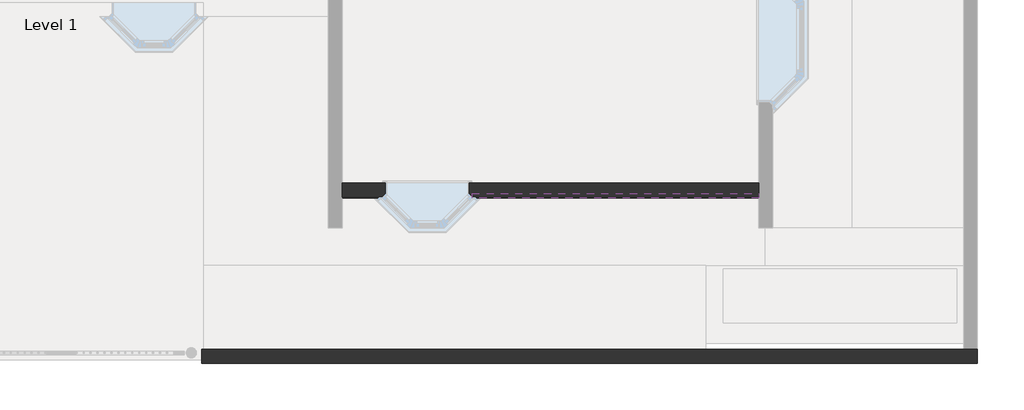
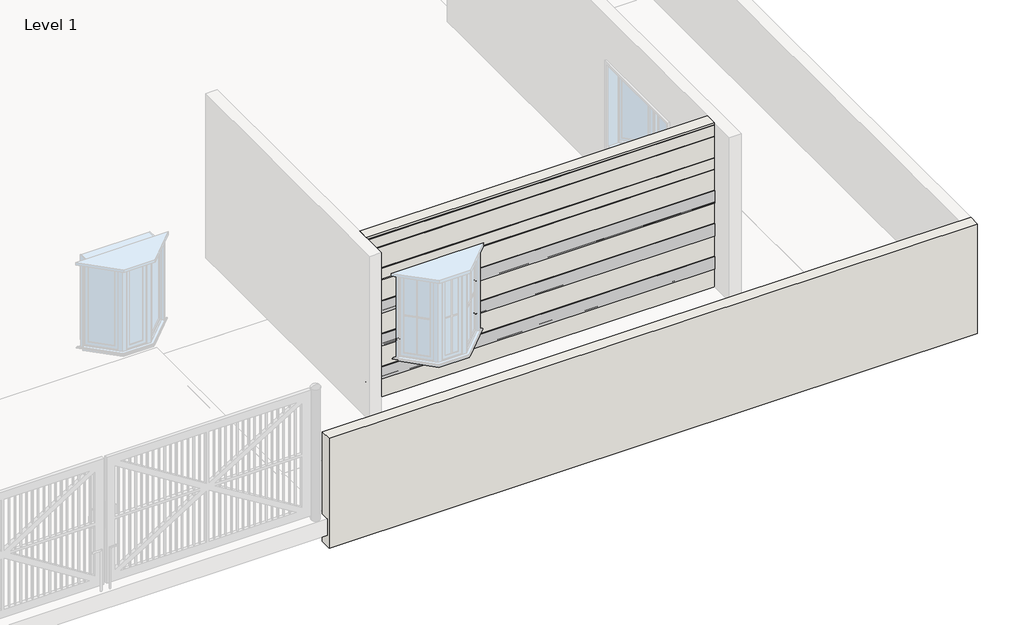
# One storey, part 2 of 5: 3 proxies, 2 walls.
"""IFC4 building model written with IfcOpenShell, lengths in millimetres."""

from ifc_helpers import new_model, si_unit, point, frame, frame_2d, origin, place, context, project, spatial, polyline, circle_curve, ellipse_curve, trimmed, segment, composite_curve, outline, extrude, faceted_brep, element, save
from ifc_brep_helpers import plane_surface, cylinder_surface, revolved_surface, advanced_brep

model = new_model("IFC4")

# Units and contexts
model_context = context("Model", 3, world=origin())
ifc_project = project(units=[si_unit("LENGTHUNIT", "METRE", prefix="MILLI")], contexts=[model_context])

# Site, building, storey
site = spatial("IfcSite", under=ifc_project)
building = spatial("IfcBuilding", under=site)
storey = spatial("IfcBuildingStorey", under=building, Name="Level 1", Elevation=0.0)

# Proxies
placement = place(None, origin())
element("IfcBuildingElementProxy", 1, Name="Reveal", ObjectType="Reveal", at=placement, inside=storey, context=model_context, shape_type="SweptSolid", body=[
    extrude(outline(composite_curve([segment(polyline([(-10015.9757973, 571.5), (-9952.7297973, 571.5), (-9952.7297973, 570.1203242)]), True, "CONTINUOUS"), segment(trimmed(circle_curve(frame_2d((-9957.9748973, 570.1203242)), 5.2451), [point((-9952.7297973, 570.1203242))], [point((-9957.1126065, 564.9465897))], False, "CARTESIAN"), True, "CONTINUOUS"), segment(polyline([(-9957.1126065, 564.9465897), (-9980.7332973, 561.0098), (-9999.9711789, 557.80348)]), True, "CONTINUOUS"), segment(trimmed(circle_curve(frame_2d((-9998.2465973, 547.456011)), 10.4902), [point((-9999.9711789, 557.80348))], [point((-10008.7367973, 547.456011))], True, "CARTESIAN"), True, "CONTINUOUS"), segment(polyline([(-10008.7367973, 547.456011), (-10008.7367973, 366.943989)]), True, "CONTINUOUS"), segment(trimmed(circle_curve(frame_2d((-9998.2465973, 366.943989)), 10.4902), [point((-10008.7367973, 366.943989))], [point((-9999.9711789, 356.59652))], True, "CARTESIAN"), True, "CONTINUOUS"), segment(polyline([(-9999.9711789, 356.59652), (-9980.7332973, 353.3902), (-9957.1126065, 349.4534103)]), True, "CONTINUOUS"), segment(trimmed(circle_curve(frame_2d((-9957.9748973, 344.2796758)), 5.2451), [point((-9957.1126065, 349.4534103))], [point((-9952.7297973, 344.2796758))], False, "CARTESIAN"), True, "CONTINUOUS"), segment(polyline([(-9952.7297973, 344.2796758), (-9952.7297973, 342.9), (-10015.9757973, 342.9), (-10015.9757973, 571.5)]), True, "CONTINUOUS")], self_intersect=False)), frame((-43545.7380314, 0.0, 0.0), z_axis=(1.0, 0.0, 0.0), x_axis=(0.0, 1.0, 0.0)), (0.0, 0.0, 1.0), 6096.0),
])
element("IfcBuildingElementProxy", 2, Name="Reveal", ObjectType="Reveal", at=placement, inside=storey, context=model_context, shape_type="SweptSolid", body=[
    extrude(outline(composite_curve([segment(polyline([(-10015.9757973, 1181.1), (-9952.7297973, 1181.1), (-9952.7297973, 1179.7203242)]), True, "CONTINUOUS"), segment(trimmed(circle_curve(frame_2d((-9957.9748973, 1179.7203242)), 5.2451), [point((-9952.7297973, 1179.7203242))], [point((-9957.1126065, 1174.5465897))], False, "CARTESIAN"), True, "CONTINUOUS"), segment(polyline([(-9957.1126065, 1174.5465897), (-9980.7332973, 1170.6098), (-9999.9711789, 1167.40348)]), True, "CONTINUOUS"), segment(trimmed(circle_curve(frame_2d((-9998.2465973, 1157.056011)), 10.4902), [point((-9999.9711789, 1167.40348))], [point((-10008.7367973, 1157.056011))], True, "CARTESIAN"), True, "CONTINUOUS"), segment(polyline([(-10008.7367973, 1157.056011), (-10008.7367973, 976.543989)]), True, "CONTINUOUS"), segment(trimmed(circle_curve(frame_2d((-9998.2465973, 976.543989)), 10.4902), [point((-10008.7367973, 976.543989))], [point((-9999.9711789, 966.19652))], True, "CARTESIAN"), True, "CONTINUOUS"), segment(polyline([(-9999.9711789, 966.19652), (-9980.7332973, 962.9902), (-9957.1126065, 959.0534103)]), True, "CONTINUOUS"), segment(trimmed(circle_curve(frame_2d((-9957.9748973, 953.8796758)), 5.2451), [point((-9957.1126065, 959.0534103))], [point((-9952.7297973, 953.8796758))], False, "CARTESIAN"), True, "CONTINUOUS"), segment(polyline([(-9952.7297973, 953.8796758), (-9952.7297973, 952.5), (-10015.9757973, 952.5), (-10015.9757973, 1181.1)]), True, "CONTINUOUS")], self_intersect=False)), frame((-41642.1466227, 0.0, 0.0), z_axis=(1.0, 0.0, 0.0), x_axis=(0.0, 1.0, 0.0)), (0.0, 0.0, 1.0), 4192.4085913),
    extrude(outline(composite_curve([segment(polyline([(-10015.9757973, 1181.1), (-9952.7297973, 1181.1), (-9952.7297973, 1179.7203242)]), True, "CONTINUOUS"), segment(trimmed(circle_curve(frame_2d((-9957.9748973, 1179.7203242)), 5.2451), [point((-9952.7297973, 1179.7203242))], [point((-9957.1126065, 1174.5465897))], False, "CARTESIAN"), True, "CONTINUOUS"), segment(polyline([(-9957.1126065, 1174.5465897), (-9980.7332973, 1170.6098), (-9999.9711789, 1167.40348)]), True, "CONTINUOUS"), segment(trimmed(circle_curve(frame_2d((-9998.2465973, 1157.056011)), 10.4902), [point((-9999.9711789, 1167.40348))], [point((-10008.7367973, 1157.056011))], True, "CARTESIAN"), True, "CONTINUOUS"), segment(polyline([(-10008.7367973, 1157.056011), (-10008.7367973, 976.543989)]), True, "CONTINUOUS"), segment(trimmed(circle_curve(frame_2d((-9998.2465973, 976.543989)), 10.4902), [point((-10008.7367973, 976.543989))], [point((-9999.9711789, 966.19652))], True, "CARTESIAN"), True, "CONTINUOUS"), segment(polyline([(-9999.9711789, 966.19652), (-9980.7332973, 962.9902), (-9957.1126065, 959.0534103)]), True, "CONTINUOUS"), segment(trimmed(circle_curve(frame_2d((-9957.9748973, 953.8796758)), 5.2451), [point((-9957.1126065, 959.0534103))], [point((-9952.7297973, 953.8796758))], False, "CARTESIAN"), True, "CONTINUOUS"), segment(polyline([(-9952.7297973, 953.8796758), (-9952.7297973, 952.5), (-10015.9757973, 952.5), (-10015.9757973, 1181.1)]), True, "CONTINUOUS")], self_intersect=False)), frame((-43545.7380314, 0.0, 0.0), z_axis=(1.0, 0.0, 0.0), x_axis=(0.0, 1.0, 0.0)), (0.0, 0.0, 1.0), 585.6085913),
])
element("IfcBuildingElementProxy", 3, Name="Reveal", ObjectType="Reveal", at=placement, inside=storey, context=model_context, shape_type="SweptSolid", body=[
    extrude(outline(composite_curve([segment(polyline([(-10015.9757973, 1790.7), (-9952.7297973, 1790.7), (-9952.7297973, 1789.3203242)]), True, "CONTINUOUS"), segment(trimmed(circle_curve(frame_2d((-9957.9748973, 1789.3203242)), 5.2451), [point((-9952.7297973, 1789.3203242))], [point((-9957.1126065, 1784.1465897))], False, "CARTESIAN"), True, "CONTINUOUS"), segment(polyline([(-9957.1126065, 1784.1465897), (-9980.7332973, 1780.2098), (-9999.9711789, 1777.00348)]), True, "CONTINUOUS"), segment(trimmed(circle_curve(frame_2d((-9998.2465973, 1766.656011)), 10.4902), [point((-9999.9711789, 1777.00348))], [point((-10008.7367973, 1766.656011))], True, "CARTESIAN"), True, "CONTINUOUS"), segment(polyline([(-10008.7367973, 1766.656011), (-10008.7367973, 1586.143989)]), True, "CONTINUOUS"), segment(trimmed(circle_curve(frame_2d((-9998.2465973, 1586.143989)), 10.4902), [point((-10008.7367973, 1586.143989))], [point((-9999.9711789, 1575.79652))], True, "CARTESIAN"), True, "CONTINUOUS"), segment(polyline([(-9999.9711789, 1575.79652), (-9980.7332973, 1572.5902), (-9957.1126065, 1568.6534103)]), True, "CONTINUOUS"), segment(trimmed(circle_curve(frame_2d((-9957.9748973, 1563.4796758)), 5.2451), [point((-9957.1126065, 1568.6534103))], [point((-9952.7297973, 1563.4796758))], False, "CARTESIAN"), True, "CONTINUOUS"), segment(polyline([(-9952.7297973, 1563.4796758), (-9952.7297973, 1562.1), (-10015.9757973, 1562.1), (-10015.9757973, 1790.7)]), True, "CONTINUOUS")], self_intersect=False)), frame((-41642.1466227, 0.0, 0.0), z_axis=(1.0, 0.0, 0.0), x_axis=(0.0, 1.0, 0.0)), (0.0, 0.0, 1.0), 4192.4085913),
    extrude(outline(composite_curve([segment(polyline([(-10015.9757973, 1790.7), (-9952.7297973, 1790.7), (-9952.7297973, 1789.3203242)]), True, "CONTINUOUS"), segment(trimmed(circle_curve(frame_2d((-9957.9748973, 1789.3203242)), 5.2451), [point((-9952.7297973, 1789.3203242))], [point((-9957.1126065, 1784.1465897))], False, "CARTESIAN"), True, "CONTINUOUS"), segment(polyline([(-9957.1126065, 1784.1465897), (-9980.7332973, 1780.2098), (-9999.9711789, 1777.00348)]), True, "CONTINUOUS"), segment(trimmed(circle_curve(frame_2d((-9998.2465973, 1766.656011)), 10.4902), [point((-9999.9711789, 1777.00348))], [point((-10008.7367973, 1766.656011))], True, "CARTESIAN"), True, "CONTINUOUS"), segment(polyline([(-10008.7367973, 1766.656011), (-10008.7367973, 1586.143989)]), True, "CONTINUOUS"), segment(trimmed(circle_curve(frame_2d((-9998.2465973, 1586.143989)), 10.4902), [point((-10008.7367973, 1586.143989))], [point((-9999.9711789, 1575.79652))], True, "CARTESIAN"), True, "CONTINUOUS"), segment(polyline([(-9999.9711789, 1575.79652), (-9980.7332973, 1572.5902), (-9957.1126065, 1568.6534103)]), True, "CONTINUOUS"), segment(trimmed(circle_curve(frame_2d((-9957.9748973, 1563.4796758)), 5.2451), [point((-9957.1126065, 1568.6534103))], [point((-9952.7297973, 1563.4796758))], False, "CARTESIAN"), True, "CONTINUOUS"), segment(polyline([(-9952.7297973, 1563.4796758), (-9952.7297973, 1562.1), (-10015.9757973, 1562.1), (-10015.9757973, 1790.7)]), True, "CONTINUOUS")], self_intersect=False)), frame((-43545.7380314, 0.0, 0.0), z_axis=(1.0, 0.0, 0.0), x_axis=(0.0, 1.0, 0.0)), (0.0, 0.0, 1.0), 585.6085913),
])

# Walls
element("IfcWall", 4, ObjectType="OUTER WALL 8\"", at=placement, inside=storey, context=model_context, shape_type="AdvancedBrep", body=[
    advanced_brep(
    [(-43545.7380314, -10001.0913973, 0.0), (-37449.7380314, -10001.0913973, 0.0), (-37449.7380314, -10001.0913973, 342.9), (-43545.7380314, -10001.0913973, 342.9), (-37449.7380314, -10001.0913973, 3048.0), (-43545.7380314, -10001.0913973, 3048.0), (-43545.7380314, -10001.0913973, 3009.9), (-37449.7380314, -10001.0913973, 3009.9), (-41642.1466227, -10001.0913973, 609.6), (-42960.1294401, -10001.0913973, 609.6), (-42960.1294401, -10001.0913973, 952.5), (-43545.7380314, -10001.0913973, 952.5), (-43545.7380314, -10001.0913973, 571.5), (-37449.7380314, -10001.0913973, 571.5), (-37449.7380314, -10001.0913973, 952.5), (-41642.1466227, -10001.0913973, 952.5), (-37449.7380314, -10001.0913973, 356.84689), (-37449.7380314, -10001.0913973, 557.55311), (-43545.7380314, -10001.0913973, 557.55311), (-43545.7380314, -10001.0913973, 356.84689), (-43545.7380314, -10001.0913973, 1167.15311), (-43545.7380314, -10001.0913973, 966.44689), (-42960.1294401, -10001.0913973, 966.44689), (-42960.1294401, -10001.0913973, 1167.15311), (-37449.7380314, -10001.0913973, 966.44689), (-37449.7380314, -10001.0913973, 1167.15311), (-41642.1466227, -10001.0913973, 1167.15311), (-41642.1466227, -10001.0913973, 966.44689), (-41642.1466227, -10001.0913973, 1181.1), (-37449.7380314, -10001.0913973, 1181.1), (-37449.7380314, -10001.0913973, 1562.1), (-41642.1466227, -10001.0913973, 1562.1), (-43545.7380314, -10001.0913973, 1181.1), (-42960.1294401, -10001.0913973, 1181.1), (-42960.1294401, -10001.0913973, 1562.1), (-43545.7380314, -10001.0913973, 1562.1), (-43545.7380314, -10001.0913973, 1776.75311), (-43545.7380314, -10001.0913973, 1576.04689), (-42960.1294401, -10001.0913973, 1576.04689), (-42960.1294401, -10001.0913973, 1776.75311), (-41642.1466227, -10001.0913973, 1776.75311), (-41642.1466227, -10001.0913973, 1576.04689), (-37449.7380314, -10001.0913973, 1576.04689), (-37449.7380314, -10001.0913973, 1776.75311), (-41642.1466227, -10001.0913973, 1790.7), (-37449.7380314, -10001.0913973, 1790.7), (-37449.7380314, -10001.0913973, 2171.7), (-41642.1466227, -10001.0913973, 2171.7), (-43545.7380314, -10001.0913973, 1790.7), (-42960.1294401, -10001.0913973, 1790.7), (-42960.1294401, -10001.0913973, 2171.7), (-43545.7380314, -10001.0913973, 2171.7), (-43545.7380314, -10001.0913973, 2386.35311), (-43545.7380314, -10001.0913973, 2185.64689), (-37449.7380314, -10001.0913973, 2185.64689), (-37449.7380314, -10001.0913973, 2386.35311), (-43545.7380314, -10001.0913973, 2400.3), (-37449.7380314, -10001.0913973, 2400.3), (-37449.7380314, -10001.0913973, 2781.3), (-43545.7380314, -10001.0913973, 2781.3), (-43545.7380314, -10001.0913973, 2995.95311), (-43545.7380314, -10001.0913973, 2795.24689), (-37449.7380314, -10001.0913973, 2795.24689), (-37449.7380314, -10001.0913973, 2995.95311), (-37449.7380314, -9797.8913973, 0.0), (-43545.7380314, -9797.8913973, 0.0), (-43545.7380314, -9797.8913973, 3048.0), (-37449.7380314, -9797.8913973, 3048.0), (-41691.5380314, -9797.8913973, 2184.4), (-42910.7380314, -9797.8913973, 2184.4), (-42910.7380314, -9797.8913973, 609.6), (-41691.5380314, -9797.8913973, 609.6), (-43545.7380314, -9952.7297973, 342.9), (-43545.7380314, -9952.7297973, 344.2796758), (-43545.7380314, -9957.1126065, 349.4534103), (-43545.7380314, -9999.9711789, 356.59652), (-43545.7380314, -9999.9711789, 557.80348), (-43545.7380314, -9957.1126065, 564.9465897), (-43545.7380314, -9952.7297973, 570.1203242), (-43545.7380314, -9952.7297973, 571.5), (-43545.7380314, -9952.7297973, 952.5), (-43545.7380314, -9952.7297973, 953.8796758), (-43545.7380314, -9957.1126065, 959.0534103), (-43545.7380314, -9999.9711789, 966.19652), (-43545.7380314, -9999.9711789, 1167.40348), (-43545.7380314, -9957.1126065, 1174.5465897), (-43545.7380314, -9952.7297973, 1179.7203242), (-43545.7380314, -9952.7297973, 1181.1), (-43545.7380314, -9952.7297973, 1562.1), (-43545.7380314, -9952.7297973, 1563.4796758), (-43545.7380314, -9957.1126065, 1568.6534103), (-43545.7380314, -9999.9711789, 1575.79652), (-43545.7380314, -9999.9711789, 1777.00348), (-43545.7380314, -9957.1126065, 1784.1465897), (-43545.7380314, -9952.7297973, 1789.3203242), (-43545.7380314, -9952.7297973, 1790.7), (-43545.7380314, -9952.7297973, 2171.7), (-43545.7380314, -9952.7297973, 2173.0796758), (-43545.7380314, -9957.1126065, 2178.2534103), (-43545.7380314, -9999.9711789, 2185.39652), (-43545.7380314, -9999.9711789, 2386.60348), (-43545.7380314, -9957.1126065, 2393.7465897), (-43545.7380314, -9952.7297973, 2398.9203242), (-43545.7380314, -9952.7297973, 2400.3), (-43545.7380314, -9952.7297973, 2781.3), (-43545.7380314, -9952.7297973, 2782.6796758), (-43545.7380314, -9957.1126065, 2787.8534103), (-43545.7380314, -9999.9711789, 2794.99652), (-43545.7380314, -9999.9711789, 2996.20348), (-43545.7380314, -9957.1126065, 3003.3465897), (-43545.7380314, -9952.7297973, 3008.5203242), (-43545.7380314, -9952.7297973, 3009.9), (-37449.7380314, -9952.7297973, 3009.9), (-37449.7380314, -9952.7297973, 3008.5203242), (-37449.7380314, -9957.1126065, 3003.3465897), (-37449.7380314, -9999.9711789, 2996.20348), (-37449.7380314, -9999.9711789, 2794.99652), (-37449.7380314, -9957.1126065, 2787.8534103), (-37449.7380314, -9952.7297973, 2782.6796758), (-37449.7380314, -9952.7297973, 2781.3), (-37449.7380314, -9952.7297973, 2400.3), (-37449.7380314, -9952.7297973, 2398.9203242), (-37449.7380314, -9957.1126065, 2393.7465897), (-37449.7380314, -9999.9711789, 2386.60348), (-37449.7380314, -9999.9711789, 2185.39652), (-37449.7380314, -9957.1126065, 2178.2534103), (-37449.7380314, -9952.7297973, 2173.0796758), (-37449.7380314, -9952.7297973, 2171.7), (-37449.7380314, -9952.7297973, 1790.7), (-37449.7380314, -9952.7297973, 1789.3203242), (-37449.7380314, -9957.1126065, 1784.1465897), (-37449.7380314, -9999.9711789, 1777.00348), (-37449.7380314, -9999.9711789, 1575.79652), (-37449.7380314, -9957.1126065, 1568.6534103), (-37449.7380314, -9952.7297973, 1563.4796758), (-37449.7380314, -9952.7297973, 1562.1), (-37449.7380314, -9952.7297973, 1181.1), (-37449.7380314, -9952.7297973, 1179.7203242), (-37449.7380314, -9957.1126065, 1174.5465897), (-37449.7380314, -9999.9711789, 1167.40348), (-37449.7380314, -9999.9711789, 966.19652), (-37449.7380314, -9957.1126065, 959.0534103), (-37449.7380314, -9952.7297973, 953.8796758), (-37449.7380314, -9952.7297973, 952.5), (-37449.7380314, -9952.7297973, 571.5), (-37449.7380314, -9952.7297973, 570.1203242), (-37449.7380314, -9957.1126065, 564.9465897), (-37449.7380314, -9999.9711789, 557.80348), (-37449.7380314, -9999.9711789, 356.59652), (-37449.7380314, -9957.1126065, 349.4534103), (-37449.7380314, -9952.7297973, 344.2796758), (-37449.7380314, -9952.7297973, 342.9), (-42910.7380314, -9951.6999886, 2184.4), (-41691.5380314, -9951.6999886, 2184.4), (-41649.2459493, -9993.9920708, 2184.4), (-42953.0301136, -9993.9920708, 2184.4), (-41691.5380314, -9951.6999886, 609.6), (-42910.7380314, -9951.6999886, 609.6), (-42916.1506493, -9957.1126065, 2178.2534103), (-42911.7678401, -9952.7297973, 2173.0796758), (-42911.7678401, -9952.7297973, 2171.7), (-41690.5082227, -9952.7297973, 2171.7), (-41690.5082227, -9952.7297973, 2173.0796758), (-41686.1254136, -9957.1126065, 2178.2534103), (-41642.1466227, -9952.7297973, 1179.7203242), (-41642.1466227, -9952.7297973, 1181.1), (-41642.1466227, -9999.9711789, 1167.40348), (-41642.1466227, -9957.1126065, 1174.5465897), (-41642.1466227, -9957.1126065, 959.0534103), (-41642.1466227, -9999.9711789, 966.19652), (-41642.1466227, -9952.7297973, 952.5), (-41642.1466227, -9952.7297973, 953.8796758), (-42960.1294401, -9952.7297973, 953.8796758), (-42960.1294401, -9952.7297973, 952.5), (-42960.1294401, -9999.9711789, 966.19652), (-42960.1294401, -9957.1126065, 959.0534103), (-42960.1294401, -9957.1126065, 1174.5465897), (-42960.1294401, -9999.9711789, 1167.40348), (-42960.1294401, -9952.7297973, 1181.1), (-42960.1294401, -9952.7297973, 1179.7203242), (-41642.1466227, -9952.7297973, 1789.3203242), (-41642.1466227, -9952.7297973, 1790.7), (-41642.1466227, -9999.9711789, 1777.00348), (-41642.1466227, -9957.1126065, 1784.1465897), (-41642.1466227, -9957.1126065, 1568.6534103), (-41642.1466227, -9999.9711789, 1575.79652), (-41642.1466227, -9952.7297973, 1562.1), (-41642.1466227, -9952.7297973, 1563.4796758), (-42960.1294401, -9952.7297973, 1563.4796758), (-42960.1294401, -9952.7297973, 1562.1), (-42960.1294401, -9999.9711789, 1575.79652), (-42960.1294401, -9957.1126065, 1568.6534103), (-42960.1294401, -9957.1126065, 1784.1465897), (-42960.1294401, -9999.9711789, 1777.00348), (-42960.1294401, -9952.7297973, 1790.7), (-42960.1294401, -9952.7297973, 1789.3203242)],
    [
        (0, 1),
        (1, 2),
        (2, 3),
        (3, 0),
        (4, 5),
        (5, 6),
        (6, 7),
        (7, 4),
        (8, 9),
        (9, 10),
        (10, 11),
        (11, 12),
        (12, 13),
        (13, 14),
        (14, 15),
        (15, 8),
        (16, 17),
        (17, 18),
        (18, 19),
        (19, 16),
        (20, 21),
        (21, 22),
        (22, 23),
        (23, 20),
        (24, 25),
        (25, 26),
        (26, 27),
        (27, 24),
        (28, 29),
        (29, 30),
        (30, 31),
        (31, 28),
        (32, 33),
        (33, 34),
        (34, 35),
        (35, 32),
        (36, 37),
        (37, 38),
        (38, 39),
        (39, 36),
        (40, 41),
        (41, 42),
        (42, 43),
        (43, 40),
        (44, 45),
        (45, 46),
        (46, 47),
        (47, 44),
        (48, 49),
        (49, 50),
        (50, 51),
        (51, 48),
        (52, 53),
        (53, 54),
        (54, 55),
        (55, 52),
        (56, 57),
        (57, 58),
        (58, 59),
        (59, 56),
        (60, 61),
        (61, 62),
        (62, 63),
        (63, 60),
        (64, 65),
        (65, 66),
        (66, 67),
        (67, 64),
        (68, 69),
        (69, 70),
        (70, 71),
        (71, 68),
        (0, 65),
        (64, 1),
        (4, 67),
        (66, 5),
        (3, 72),
        (72, 73),
        (73, 74, circle_curve(frame((-43545.7380314, -9957.9748973, 344.2796758), z_axis=(1.0, 0.0, 0.0), x_axis=(0.0, 1.0, 0.0)), 5.2451)),
        (74, 75),
        (75, 19, circle_curve(frame((-43545.7380314, -9998.2465973, 366.943989), z_axis=(-1.0, 0.0, 0.0), x_axis=(0.0, 1.0, 0.0)), 10.4902)),
        (18, 76, circle_curve(frame((-43545.7380314, -9998.2465973, 547.456011), z_axis=(-1.0, 0.0, 0.0), x_axis=(0.0, 1.0, 0.0)), 10.4902)),
        (76, 77),
        (77, 78, circle_curve(frame((-43545.7380314, -9957.9748973, 570.1203242), z_axis=(1.0, 0.0, 0.0), x_axis=(0.0, 1.0, 0.0)), 5.2451)),
        (78, 79),
        (79, 12),
        (11, 80),
        (80, 81),
        (81, 82, circle_curve(frame((-43545.7380314, -9957.9748973, 953.8796758), z_axis=(1.0, 0.0, 0.0), x_axis=(0.0, 1.0, 0.0)), 5.2451)),
        (82, 83),
        (83, 21, circle_curve(frame((-43545.7380314, -9998.2465973, 976.543989), z_axis=(-1.0, 0.0, 0.0), x_axis=(0.0, 1.0, 0.0)), 10.4902)),
        (20, 84, circle_curve(frame((-43545.7380314, -9998.2465973, 1157.056011), z_axis=(-1.0, 0.0, 0.0), x_axis=(0.0, 1.0, 0.0)), 10.4902)),
        (84, 85),
        (85, 86, circle_curve(frame((-43545.7380314, -9957.9748973, 1179.7203242), z_axis=(1.0, 0.0, 0.0), x_axis=(0.0, 1.0, 0.0)), 5.2451)),
        (86, 87),
        (87, 32),
        (35, 88),
        (88, 89),
        (89, 90, circle_curve(frame((-43545.7380314, -9957.9748973, 1563.4796758), z_axis=(1.0, 0.0, 0.0), x_axis=(0.0, 1.0, 0.0)), 5.2451)),
        (90, 91),
        (91, 37, circle_curve(frame((-43545.7380314, -9998.2465973, 1586.143989), z_axis=(-1.0, 0.0, 0.0), x_axis=(0.0, 1.0, 0.0)), 10.4902)),
        (36, 92, circle_curve(frame((-43545.7380314, -9998.2465973, 1766.656011), z_axis=(-1.0, 0.0, 0.0), x_axis=(0.0, 1.0, 0.0)), 10.4902)),
        (92, 93),
        (93, 94, circle_curve(frame((-43545.7380314, -9957.9748973, 1789.3203242), z_axis=(1.0, 0.0, 0.0), x_axis=(0.0, 1.0, 0.0)), 5.2451)),
        (94, 95),
        (95, 48),
        (51, 96),
        (96, 97),
        (97, 98, circle_curve(frame((-43545.7380314, -9957.9748973, 2173.0796758), z_axis=(1.0, 0.0, 0.0), x_axis=(0.0, 1.0, 0.0)), 5.2451)),
        (98, 99),
        (99, 53, circle_curve(frame((-43545.7380314, -9998.2465973, 2195.743989), z_axis=(-1.0, 0.0, 0.0), x_axis=(0.0, 1.0, 0.0)), 10.4902)),
        (52, 100, circle_curve(frame((-43545.7380314, -9998.2465973, 2376.256011), z_axis=(-1.0, 0.0, 0.0), x_axis=(0.0, 1.0, 0.0)), 10.4902)),
        (100, 101),
        (101, 102, circle_curve(frame((-43545.7380314, -9957.9748973, 2398.9203242), z_axis=(1.0, 0.0, 0.0), x_axis=(0.0, 1.0, 0.0)), 5.2451)),
        (102, 103),
        (103, 56),
        (59, 104),
        (104, 105),
        (105, 106, circle_curve(frame((-43545.7380314, -9957.9748973, 2782.6796758), z_axis=(1.0, 0.0, 0.0), x_axis=(0.0, 1.0, 0.0)), 5.2451)),
        (106, 107),
        (107, 61, circle_curve(frame((-43545.7380314, -9998.2465973, 2805.343989), z_axis=(-1.0, 0.0, 0.0), x_axis=(0.0, 1.0, 0.0)), 10.4902)),
        (60, 108, circle_curve(frame((-43545.7380314, -9998.2465973, 2985.856011), z_axis=(-1.0, 0.0, 0.0), x_axis=(0.0, 1.0, 0.0)), 10.4902)),
        (108, 109),
        (109, 110, circle_curve(frame((-43545.7380314, -9957.9748973, 3008.5203242), z_axis=(1.0, 0.0, 0.0), x_axis=(0.0, 1.0, 0.0)), 5.2451)),
        (110, 111),
        (111, 6),
        (7, 112),
        (112, 113),
        (113, 114, circle_curve(frame((-37449.7380314, -9957.9748973, 3008.5203242), z_axis=(-1.0, 0.0, 0.0), x_axis=(0.0, 1.0, 0.0)), 5.2451)),
        (114, 115),
        (115, 63, circle_curve(frame((-37449.7380314, -9998.2465973, 2985.856011), z_axis=(1.0, 0.0, 0.0), x_axis=(0.0, 1.0, 0.0)), 10.4902)),
        (62, 116, circle_curve(frame((-37449.7380314, -9998.2465973, 2805.343989), z_axis=(1.0, 0.0, 0.0), x_axis=(0.0, 1.0, 0.0)), 10.4902)),
        (116, 117),
        (117, 118, circle_curve(frame((-37449.7380314, -9957.9748973, 2782.6796758), z_axis=(-1.0, 0.0, 0.0), x_axis=(0.0, 1.0, 0.0)), 5.2451)),
        (118, 119),
        (119, 58),
        (57, 120),
        (120, 121),
        (121, 122, circle_curve(frame((-37449.7380314, -9957.9748973, 2398.9203242), z_axis=(-1.0, 0.0, 0.0), x_axis=(0.0, 1.0, 0.0)), 5.2451)),
        (122, 123),
        (123, 55, circle_curve(frame((-37449.7380314, -9998.2465973, 2376.256011), z_axis=(1.0, 0.0, 0.0), x_axis=(0.0, 1.0, 0.0)), 10.4902)),
        (54, 124, circle_curve(frame((-37449.7380314, -9998.2465973, 2195.743989), z_axis=(1.0, 0.0, 0.0), x_axis=(0.0, 1.0, 0.0)), 10.4902)),
        (124, 125),
        (125, 126, circle_curve(frame((-37449.7380314, -9957.9748973, 2173.0796758), z_axis=(-1.0, 0.0, 0.0), x_axis=(0.0, 1.0, 0.0)), 5.2451)),
        (126, 127),
        (127, 46),
        (45, 128),
        (128, 129),
        (129, 130, circle_curve(frame((-37449.7380314, -9957.9748973, 1789.3203242), z_axis=(-1.0, 0.0, 0.0), x_axis=(0.0, 1.0, 0.0)), 5.2451)),
        (130, 131),
        (131, 43, circle_curve(frame((-37449.7380314, -9998.2465973, 1766.656011), z_axis=(1.0, 0.0, 0.0), x_axis=(0.0, 1.0, 0.0)), 10.4902)),
        (42, 132, circle_curve(frame((-37449.7380314, -9998.2465973, 1586.143989), z_axis=(1.0, 0.0, 0.0), x_axis=(0.0, 1.0, 0.0)), 10.4902)),
        (132, 133),
        (133, 134, circle_curve(frame((-37449.7380314, -9957.9748973, 1563.4796758), z_axis=(-1.0, 0.0, 0.0), x_axis=(0.0, 1.0, 0.0)), 5.2451)),
        (134, 135),
        (135, 30),
        (29, 136),
        (136, 137),
        (137, 138, circle_curve(frame((-37449.7380314, -9957.9748973, 1179.7203242), z_axis=(-1.0, 0.0, 0.0), x_axis=(0.0, 1.0, 0.0)), 5.2451)),
        (138, 139),
        (139, 25, circle_curve(frame((-37449.7380314, -9998.2465973, 1157.056011), z_axis=(1.0, 0.0, 0.0), x_axis=(0.0, 1.0, 0.0)), 10.4902)),
        (24, 140, circle_curve(frame((-37449.7380314, -9998.2465973, 976.543989), z_axis=(1.0, 0.0, 0.0), x_axis=(0.0, 1.0, 0.0)), 10.4902)),
        (140, 141),
        (141, 142, circle_curve(frame((-37449.7380314, -9957.9748973, 953.8796758), z_axis=(-1.0, 0.0, 0.0), x_axis=(0.0, 1.0, 0.0)), 5.2451)),
        (142, 143),
        (143, 14),
        (13, 144),
        (144, 145),
        (145, 146, circle_curve(frame((-37449.7380314, -9957.9748973, 570.1203242), z_axis=(-1.0, 0.0, 0.0), x_axis=(0.0, 1.0, 0.0)), 5.2451)),
        (146, 147),
        (147, 17, circle_curve(frame((-37449.7380314, -9998.2465973, 547.456011), z_axis=(1.0, 0.0, 0.0), x_axis=(0.0, 1.0, 0.0)), 10.4902)),
        (16, 148, circle_curve(frame((-37449.7380314, -9998.2465973, 366.943989), z_axis=(1.0, 0.0, 0.0), x_axis=(0.0, 1.0, 0.0)), 10.4902)),
        (148, 149),
        (149, 150, circle_curve(frame((-37449.7380314, -9957.9748973, 344.2796758), z_axis=(-1.0, 0.0, 0.0), x_axis=(0.0, 1.0, 0.0)), 5.2451)),
        (150, 151),
        (151, 2),
        (152, 69),
        (68, 153),
        (153, 154),
        (154, 155),
        (155, 152),
        (156, 71),
        (70, 157),
        (157, 9),
        (8, 156),
        (156, 153),
        (152, 157),
        (155, 158),
        (158, 159, ellipse_curve(frame((-42917.0129401, -9957.9748973, 2173.0796758), z_axis=(-0.7071067811865462, 0.7071067811865489, 0.0), x_axis=(-0.7071067811865488, -0.7071067811865462, 0.0)), 7.4176916, 5.2451)),
        (159, 160),
        (160, 50),
        (49, 39),
        (38, 34),
        (33, 23),
        (22, 10),
        (15, 27),
        (26, 28),
        (31, 41),
        (40, 44),
        (47, 161),
        (161, 162),
        (162, 163, ellipse_curve(frame((-41685.2631227, -9957.9748973, 2173.0796758), z_axis=(0.707106781186551, 0.7071067811865441, 0.0), x_axis=(-0.707106781186544, 0.707106781186551, 0.0)), 7.4176916, 5.2451)),
        (163, 154),
        (79, 144),
        (78, 145),
        (77, 146),
        (76, 147),
        (75, 148),
        (74, 149),
        (73, 150),
        (72, 151),
        (164, 165),
        (165, 28),
        (26, 166, circle_curve(frame((-41642.1466227, -9998.2465973, 1157.056011), z_axis=(-1.0, 0.0, 0.0), x_axis=(0.0, 1.0, 0.0)), 10.4902)),
        (166, 167),
        (167, 164, circle_curve(frame((-41642.1466227, -9957.9748973, 1179.7203242), z_axis=(1.0, 0.0, 0.0), x_axis=(0.0, 1.0, 0.0)), 5.2451)),
        (168, 169),
        (169, 27, circle_curve(frame((-41642.1466227, -9998.2465973, 976.543989), z_axis=(-1.0, 0.0, 0.0), x_axis=(0.0, 1.0, 0.0)), 10.4902)),
        (15, 170),
        (170, 171),
        (171, 168, circle_curve(frame((-41642.1466227, -9957.9748973, 953.8796758), z_axis=(1.0, 0.0, 0.0), x_axis=(0.0, 1.0, 0.0)), 5.2451)),
        (165, 136),
        (164, 137),
        (167, 138),
        (166, 139),
        (169, 140),
        (168, 141),
        (171, 142),
        (170, 143),
        (172, 173),
        (173, 10),
        (22, 174, circle_curve(frame((-42960.1294401, -9998.2465973, 976.543989), z_axis=(1.0, 0.0, 0.0), x_axis=(0.0, 1.0, 0.0)), 10.4902)),
        (174, 175),
        (175, 172, circle_curve(frame((-42960.1294401, -9957.9748973, 953.8796758), z_axis=(-1.0, 0.0, 0.0), x_axis=(0.0, 1.0, 0.0)), 5.2451)),
        (176, 177),
        (177, 23, circle_curve(frame((-42960.1294401, -9998.2465973, 1157.056011), z_axis=(1.0, 0.0, 0.0), x_axis=(0.0, 1.0, 0.0)), 10.4902)),
        (33, 178),
        (178, 179),
        (179, 176, circle_curve(frame((-42960.1294401, -9957.9748973, 1179.7203242), z_axis=(-1.0, 0.0, 0.0), x_axis=(0.0, 1.0, 0.0)), 5.2451)),
        (87, 178),
        (86, 179),
        (85, 176),
        (84, 177),
        (83, 174),
        (82, 175),
        (81, 172),
        (80, 173),
        (180, 181),
        (181, 44),
        (40, 182, circle_curve(frame((-41642.1466227, -9998.2465973, 1766.656011), z_axis=(-1.0, 0.0, 0.0), x_axis=(0.0, 1.0, 0.0)), 10.4902)),
        (182, 183),
        (183, 180, circle_curve(frame((-41642.1466227, -9957.9748973, 1789.3203242), z_axis=(1.0, 0.0, 0.0), x_axis=(0.0, 1.0, 0.0)), 5.2451)),
        (184, 185),
        (185, 41, circle_curve(frame((-41642.1466227, -9998.2465973, 1586.143989), z_axis=(-1.0, 0.0, 0.0), x_axis=(0.0, 1.0, 0.0)), 10.4902)),
        (31, 186),
        (186, 187),
        (187, 184, circle_curve(frame((-41642.1466227, -9957.9748973, 1563.4796758), z_axis=(1.0, 0.0, 0.0), x_axis=(0.0, 1.0, 0.0)), 5.2451)),
        (181, 128),
        (180, 129),
        (183, 130),
        (182, 131),
        (185, 132),
        (184, 133),
        (187, 134),
        (186, 135),
        (188, 189),
        (189, 34),
        (38, 190, circle_curve(frame((-42960.1294401, -9998.2465973, 1586.143989), z_axis=(1.0, 0.0, 0.0), x_axis=(0.0, 1.0, 0.0)), 10.4902)),
        (190, 191),
        (191, 188, circle_curve(frame((-42960.1294401, -9957.9748973, 1563.4796758), z_axis=(-1.0, 0.0, 0.0), x_axis=(0.0, 1.0, 0.0)), 5.2451)),
        (192, 193),
        (193, 39, circle_curve(frame((-42960.1294401, -9998.2465973, 1766.656011), z_axis=(1.0, 0.0, 0.0), x_axis=(0.0, 1.0, 0.0)), 10.4902)),
        (49, 194),
        (194, 195),
        (195, 192, circle_curve(frame((-42960.1294401, -9957.9748973, 1789.3203242), z_axis=(-1.0, 0.0, 0.0), x_axis=(0.0, 1.0, 0.0)), 5.2451)),
        (95, 194),
        (94, 195),
        (93, 192),
        (92, 193),
        (91, 190),
        (90, 191),
        (89, 188),
        (88, 189),
        (103, 120),
        (102, 121),
        (101, 122),
        (100, 123),
        (99, 124),
        (98, 158),
        (163, 125),
        (97, 159),
        (162, 126),
        (96, 160),
        (161, 127),
        (111, 112),
        (110, 113),
        (109, 114),
        (108, 115),
        (107, 116),
        (106, 117),
        (105, 118),
        (104, 119),
    ],
    [
        plane_surface(frame((-43545.7380314, -10001.0913973, 0.0), z_axis=(0.0, -1.0, 0.0), x_axis=(1.0, 0.0, 0.0))),
        plane_surface(frame((-43545.7380314, -9797.8913973, 0.0), z_axis=(0.0, 1.0, 0.0), x_axis=(-1.0, 0.0, 0.0))),
        plane_surface(frame((-43647.3380314, -10001.0913973, 0.0), z_axis=(0.0, 0.0, -1.0), x_axis=(0.0, 1.0, 0.0))),
        plane_surface(frame((-37348.1380314, -10001.0913973, 3048.0), z_axis=(0.0, 0.0, 1.0), x_axis=(0.0, 1.0, 0.0))),
        plane_surface(frame((-43545.7380314, -10453.4560416, 0.0), z_axis=(-1.0, 0.0, 0.0), x_axis=(0.0, 1.0, 0.0))),
        plane_surface(frame((-37449.7380314, -10442.4509921, 0.0), z_axis=(1.0, 0.0, 0.0), x_axis=(0.0, -1.0, 0.0))),
        plane_surface(frame((-41691.5380314, -9951.6999886, 2184.4), z_axis=(0.0, 0.0, -1.0), x_axis=(0.0, 1.0, 0.0))),
        plane_surface(frame((-41691.5380314, -9951.6999886, 609.6), z_axis=(0.0, 0.0, 1.0), x_axis=(0.0, -1.0, 0.0))),
        plane_surface(frame((-41691.5380314, -9951.6999886, 2184.4), z_axis=(-1.0, 0.0, 0.0), x_axis=(0.0, 0.0, -1.0))),
        plane_surface(frame((-42910.7380314, -9797.8913973, 2184.4), z_axis=(1.0, 0.0, 0.0), x_axis=(0.0, 0.0, -1.0))),
        plane_surface(frame((-42910.7380314, -9951.6999886, 2184.4), z_axis=(0.7071067811865462, -0.7071067811865489, 0.0), x_axis=(0.0, 0.0, -1.0))),
        plane_surface(frame((-41642.1466227, -10001.0913973, 2184.4), z_axis=(-0.707106781186551, -0.7071067811865441, 0.0), x_axis=(0.0, 0.0, -1.0))),
        plane_surface(frame((-43545.7380314, -10015.9757973, 571.5), z_axis=(0.0, 0.0, -1.0), x_axis=(1.0, 0.0, 0.0))),
        plane_surface(frame((-43545.7380314, -9952.7297973, 571.5), z_axis=(0.0, -1.0, 0.0), x_axis=(1.0, 0.0, 0.0))),
        revolved_surface(polyline([(-43545.7380314, -9952.7297973, 570.1203242), (-37449.7380314, -9952.7297973, 570.1203242)]), (-43545.7380314, -9957.9748973, 570.1203242), (-1.0, 0.0, 0.0)),
        plane_surface(frame((-43545.7380314, -9980.7332973, 561.0098), z_axis=(0.0, -0.16439930721687146, 0.9863938705135048), x_axis=(1.0, 0.0, 0.0))),
        cylinder_surface(frame((-43545.7380314, -9998.2465973, 547.456011), z_axis=(1.0, 0.0, 0.0), x_axis=(0.0, 1.0, 0.0)), 10.4902),
        cylinder_surface(frame((-43545.7380314, -9998.2465973, 366.943989), z_axis=(1.0, 0.0, 0.0), x_axis=(0.0, 1.0, 0.0)), 10.4902),
        plane_surface(frame((-43545.7380314, -9980.7332973, 353.3902), z_axis=(0.0, -0.16439930721687793, -0.9863938705135037), x_axis=(1.0, 0.0, 0.0))),
        revolved_surface(polyline([(-43545.7380314, -9952.7297973, 344.2796758), (-37449.7380314, -9952.7297973, 344.2796758)]), (-43545.7380314, -9957.9748973, 344.2796758), (-1.0, 0.0, 0.0)),
        plane_surface(frame((-43545.7380314, -9952.7297973, 344.2796758), z_axis=(0.0, -1.0, 0.0), x_axis=(1.0, 0.0, 0.0))),
        plane_surface(frame((-43545.7380314, -9952.7297973, 342.9), z_axis=(0.0, 0.0, 1.0), x_axis=(1.0, 0.0, 0.0))),
        plane_surface(frame((-41642.1466227, -10001.0913973, 942.6898298), z_axis=(1.0, 0.0, 0.0), x_axis=(0.0, 1.0, 0.0))),
        plane_surface(frame((-41642.1466227, -10015.9757973, 1181.1), z_axis=(0.0, 0.0, -1.0), x_axis=(1.0, 0.0, 0.0))),
        plane_surface(frame((-41642.1466227, -9952.7297973, 1181.1), z_axis=(0.0, -1.0, 0.0), x_axis=(1.0, 0.0, 0.0))),
        revolved_surface(polyline([(-41642.1466227, -9952.7297973, 1179.7203242), (-37449.7380314, -9952.7297973, 1179.7203242)]), (-41642.1466227, -9957.9748973, 1179.7203242), (-1.0, 0.0, 0.0)),
        plane_surface(frame((-41642.1466227, -9980.7332973, 1170.6098), z_axis=(0.0, -0.16439930721687146, 0.9863938705135048), x_axis=(1.0, 0.0, 0.0))),
        cylinder_surface(frame((-41642.1466227, -9998.2465973, 1157.056011), z_axis=(1.0, 0.0, 0.0), x_axis=(0.0, 1.0, 0.0)), 10.4902),
        cylinder_surface(frame((-41642.1466227, -9998.2465973, 976.543989), z_axis=(1.0, 0.0, 0.0), x_axis=(0.0, 1.0, 0.0)), 10.4902),
        plane_surface(frame((-41642.1466227, -9980.7332973, 962.9902), z_axis=(0.0, -0.16439930721687793, -0.9863938705135037), x_axis=(1.0, 0.0, 0.0))),
        revolved_surface(polyline([(-41642.1466227, -9952.7297973, 953.8796758), (-37449.7380314, -9952.7297973, 953.8796758)]), (-41642.1466227, -9957.9748973, 953.8796758), (-1.0, 0.0, 0.0)),
        plane_surface(frame((-41642.1466227, -9952.7297973, 953.8796758), z_axis=(0.0, -1.0, 0.0), x_axis=(1.0, 0.0, 0.0))),
        plane_surface(frame((-41642.1466227, -9952.7297973, 952.5), z_axis=(0.0, 0.0, 1.0), x_axis=(1.0, 0.0, 0.0))),
        plane_surface(frame((-42960.1294401, -10001.0913973, 942.6898298), z_axis=(-1.0, 0.0, 0.0), x_axis=(0.0, 1.0, 0.0))),
        plane_surface(frame((-43545.7380314, -10015.9757973, 1181.1), z_axis=(0.0, 0.0, -1.0), x_axis=(1.0, 0.0, 0.0))),
        plane_surface(frame((-43545.7380314, -9952.7297973, 1181.1), z_axis=(0.0, -1.0, 0.0), x_axis=(1.0, 0.0, 0.0))),
        revolved_surface(polyline([(-43545.7380314, -9952.7297973, 1179.7203242), (-42960.1294401, -9952.7297973, 1179.7203242)]), (-43545.7380314, -9957.9748973, 1179.7203242), (-1.0, 0.0, 0.0)),
        plane_surface(frame((-43545.7380314, -9980.7332973, 1170.6098), z_axis=(0.0, -0.16439930721687146, 0.9863938705135048), x_axis=(1.0, 0.0, 0.0))),
        cylinder_surface(frame((-43545.7380314, -9998.2465973, 1157.056011), z_axis=(1.0, 0.0, 0.0), x_axis=(0.0, 1.0, 0.0)), 10.4902),
        cylinder_surface(frame((-43545.7380314, -9998.2465973, 976.543989), z_axis=(1.0, 0.0, 0.0), x_axis=(0.0, 1.0, 0.0)), 10.4902),
        plane_surface(frame((-43545.7380314, -9980.7332973, 962.9902), z_axis=(0.0, -0.16439930721687793, -0.9863938705135037), x_axis=(1.0, 0.0, 0.0))),
        revolved_surface(polyline([(-43545.7380314, -9952.7297973, 953.8796758), (-42960.1294401, -9952.7297973, 953.8796758)]), (-43545.7380314, -9957.9748973, 953.8796758), (-1.0, 0.0, 0.0)),
        plane_surface(frame((-43545.7380314, -9952.7297973, 953.8796758), z_axis=(0.0, -1.0, 0.0), x_axis=(1.0, 0.0, 0.0))),
        plane_surface(frame((-43545.7380314, -9952.7297973, 952.5), z_axis=(0.0, 0.0, 1.0), x_axis=(1.0, 0.0, 0.0))),
        plane_surface(frame((-41642.1466227, -10001.0913973, 1552.2898298), z_axis=(1.0, 0.0, 0.0), x_axis=(0.0, 1.0, 0.0))),
        plane_surface(frame((-41642.1466227, -10015.9757973, 1790.7), z_axis=(0.0, 0.0, -1.0), x_axis=(1.0, 0.0, 0.0))),
        plane_surface(frame((-41642.1466227, -9952.7297973, 1790.7), z_axis=(0.0, -1.0, 0.0), x_axis=(1.0, 0.0, 0.0))),
        revolved_surface(polyline([(-41642.1466227, -9952.7297973, 1789.3203242), (-37449.7380314, -9952.7297973, 1789.3203242)]), (-41642.1466227, -9957.9748973, 1789.3203242), (-1.0, 0.0, 0.0)),
        plane_surface(frame((-41642.1466227, -9980.7332973, 1780.2098), z_axis=(0.0, -0.16439930721687146, 0.9863938705135048), x_axis=(1.0, 0.0, 0.0))),
        cylinder_surface(frame((-41642.1466227, -9998.2465973, 1766.656011), z_axis=(1.0, 0.0, 0.0), x_axis=(0.0, 1.0, 0.0)), 10.4902),
        cylinder_surface(frame((-41642.1466227, -9998.2465973, 1586.143989), z_axis=(1.0, 0.0, 0.0), x_axis=(0.0, 1.0, 0.0)), 10.4902),
        plane_surface(frame((-41642.1466227, -9980.7332973, 1572.5902), z_axis=(0.0, -0.16439930721687793, -0.9863938705135037), x_axis=(1.0, 0.0, 0.0))),
        revolved_surface(polyline([(-41642.1466227, -9952.7297973, 1563.4796758), (-37449.7380314, -9952.7297973, 1563.4796758)]), (-41642.1466227, -9957.9748973, 1563.4796758), (-1.0, 0.0, 0.0)),
        plane_surface(frame((-41642.1466227, -9952.7297973, 1563.4796758), z_axis=(0.0, -1.0, 0.0), x_axis=(1.0, 0.0, 0.0))),
        plane_surface(frame((-41642.1466227, -9952.7297973, 1562.1), z_axis=(0.0, 0.0, 1.0), x_axis=(1.0, 0.0, 0.0))),
        plane_surface(frame((-42960.1294401, -10001.0913973, 1552.2898298), z_axis=(-1.0, 0.0, 0.0), x_axis=(0.0, 1.0, 0.0))),
        plane_surface(frame((-43545.7380314, -10015.9757973, 1790.7), z_axis=(0.0, 0.0, -1.0), x_axis=(1.0, 0.0, 0.0))),
        plane_surface(frame((-43545.7380314, -9952.7297973, 1790.7), z_axis=(0.0, -1.0, 0.0), x_axis=(1.0, 0.0, 0.0))),
        revolved_surface(polyline([(-43545.7380314, -9952.7297973, 1789.3203242), (-42960.1294401, -9952.7297973, 1789.3203242)]), (-43545.7380314, -9957.9748973, 1789.3203242), (-1.0, 0.0, 0.0)),
        plane_surface(frame((-43545.7380314, -9980.7332973, 1780.2098), z_axis=(0.0, -0.16439930721687146, 0.9863938705135048), x_axis=(1.0, 0.0, 0.0))),
        cylinder_surface(frame((-43545.7380314, -9998.2465973, 1766.656011), z_axis=(1.0, 0.0, 0.0), x_axis=(0.0, 1.0, 0.0)), 10.4902),
        cylinder_surface(frame((-43545.7380314, -9998.2465973, 1586.143989), z_axis=(1.0, 0.0, 0.0), x_axis=(0.0, 1.0, 0.0)), 10.4902),
        plane_surface(frame((-43545.7380314, -9980.7332973, 1572.5902), z_axis=(0.0, -0.16439930721687793, -0.9863938705135037), x_axis=(1.0, 0.0, 0.0))),
        revolved_surface(polyline([(-43545.7380314, -9952.7297973, 1563.4796758), (-42960.1294401, -9952.7297973, 1563.4796758)]), (-43545.7380314, -9957.9748973, 1563.4796758), (-1.0, 0.0, 0.0)),
        plane_surface(frame((-43545.7380314, -9952.7297973, 1563.4796758), z_axis=(0.0, -1.0, 0.0), x_axis=(1.0, 0.0, 0.0))),
        plane_surface(frame((-43545.7380314, -9952.7297973, 1562.1), z_axis=(0.0, 0.0, 1.0), x_axis=(1.0, 0.0, 0.0))),
        plane_surface(frame((-43545.7380314, -10015.9757973, 2400.3), z_axis=(0.0, 0.0, -1.0), x_axis=(1.0, 0.0, 0.0))),
        plane_surface(frame((-43545.7380314, -9952.7297973, 2400.3), z_axis=(0.0, -1.0, 0.0), x_axis=(1.0, 0.0, 0.0))),
        revolved_surface(polyline([(-43545.7380314, -9952.7297973, 2398.9203242), (-37449.7380314, -9952.7297973, 2398.9203242)]), (-43545.7380314, -9957.9748973, 2398.9203242), (-1.0, 0.0, 0.0)),
        plane_surface(frame((-43545.7380314, -9980.7332973, 2389.8098), z_axis=(0.0, -0.16439930721687146, 0.9863938705135048), x_axis=(1.0, 0.0, 0.0))),
        cylinder_surface(frame((-43545.7380314, -9998.2465973, 2376.256011), z_axis=(1.0, 0.0, 0.0), x_axis=(0.0, 1.0, 0.0)), 10.4902),
        cylinder_surface(frame((-43545.7380314, -9998.2465973, 2195.743989), z_axis=(1.0, 0.0, 0.0), x_axis=(0.0, 1.0, 0.0)), 10.4902),
        plane_surface(frame((-43545.7380314, -9980.7332973, 2182.1902), z_axis=(0.0, -0.16439930721687793, -0.9863938705135037), x_axis=(1.0, 0.0, 0.0))),
        revolved_surface(polyline([(-43545.7380314, -9952.7297973, 2173.0796758), (-42911.76784006889, -9952.7297973, 2173.0796758)]), (-43545.7380314, -9957.9748973, 2173.0796758), (-1.0, 0.0, 0.0)),
        revolved_surface(polyline([(-41690.508222731114, -9952.7297973, 2173.0796758), (-37449.7380314, -9952.7297973, 2173.0796758)]), (-43545.7380314, -9957.9748973, 2173.0796758), (-1.0, 0.0, 0.0)),
        plane_surface(frame((-43545.7380314, -9952.7297973, 2173.0796758), z_axis=(0.0, -1.0, 0.0), x_axis=(1.0, 0.0, 0.0))),
        plane_surface(frame((-43545.7380314, -9952.7297973, 2171.7), z_axis=(0.0, 0.0, 1.0), x_axis=(1.0, 0.0, 0.0))),
        plane_surface(frame((-43545.7380314, -10015.9757973, 3009.9), z_axis=(0.0, 0.0, -1.0), x_axis=(1.0, 0.0, 0.0))),
        plane_surface(frame((-43545.7380314, -9952.7297973, 3009.9), z_axis=(0.0, -1.0, 0.0), x_axis=(1.0, 0.0, 0.0))),
        revolved_surface(polyline([(-43545.7380314, -9952.7297973, 3008.5203242), (-37449.7380314, -9952.7297973, 3008.5203242)]), (-43545.7380314, -9957.9748973, 3008.5203242), (-1.0, 0.0, 0.0)),
        plane_surface(frame((-43545.7380314, -9980.7332973, 2999.4098), z_axis=(0.0, -0.16439930721687146, 0.9863938705135048), x_axis=(1.0, 0.0, 0.0))),
        cylinder_surface(frame((-43545.7380314, -9998.2465973, 2985.856011), z_axis=(1.0, 0.0, 0.0), x_axis=(0.0, 1.0, 0.0)), 10.4902),
        cylinder_surface(frame((-43545.7380314, -9998.2465973, 2805.343989), z_axis=(1.0, 0.0, 0.0), x_axis=(0.0, 1.0, 0.0)), 10.4902),
        plane_surface(frame((-43545.7380314, -9980.7332973, 2791.7902), z_axis=(0.0, -0.16439930721687793, -0.9863938705135037), x_axis=(1.0, 0.0, 0.0))),
        revolved_surface(polyline([(-43545.7380314, -9952.7297973, 2782.6796758), (-37449.7380314, -9952.7297973, 2782.6796758)]), (-43545.7380314, -9957.9748973, 2782.6796758), (-1.0, 0.0, 0.0)),
        plane_surface(frame((-43545.7380314, -9952.7297973, 2782.6796758), z_axis=(0.0, -1.0, 0.0), x_axis=(1.0, 0.0, 0.0))),
        plane_surface(frame((-43545.7380314, -9952.7297973, 2781.3), z_axis=(0.0, 0.0, 1.0), x_axis=(1.0, 0.0, 0.0))),
    ],
    [
        (0, [[1, 2, 3, 4]]),
        (0, [[5, 6, 7, 8]]),
        (0, [[9, 10, 11, 12, 13, 14, 15, 16]]),
        (0, [[17, 18, 19, 20]]),
        (0, [[21, 22, 23, 24]]),
        (0, [[25, 26, 27, 28]]),
        (0, [[29, 30, 31, 32]]),
        (0, [[33, 34, 35, 36]]),
        (0, [[37, 38, 39, 40]]),
        (0, [[41, 42, 43, 44]]),
        (0, [[45, 46, 47, 48]]),
        (0, [[49, 50, 51, 52]]),
        (0, [[53, 54, 55, 56]]),
        (0, [[57, 58, 59, 60]]),
        (0, [[61, 62, 63, 64]]),
        (1, [[65, 66, 67, 68], [69, 70, 71, 72]]),
        (2, [[-1, 73, -65, 74]]),
        (3, [[-5, 75, -67, 76]]),
        (4, [[-76, -66, -73, -4, 77, 78, 79, 80, 81, -19, 82, 83, 84, 85, 86, -12, 87, 88, 89, 90, 91, -21, 92, 93, 94, 95, 96, -36, 97, 98, 99, 100, 101, -37, 102, 103, 104, 105, 106, -52, 107, 108, 109, 110, 111, -53, 112, 113, 114, 115, 116, -60, 117, 118, 119, 120, 121, -61, 122, 123, 124, 125, 126, -6]]),
        (5, [[-74, -68, -75, -8, 127, 128, 129, 130, 131, -63, 132, 133, 134, 135, 136, -58, 137, 138, 139, 140, 141, -55, 142, 143, 144, 145, 146, -46, 147, 148, 149, 150, 151, -43, 152, 153, 154, 155, 156, -30, 157, 158, 159, 160, 161, -25, 162, 163, 164, 165, 166, -14, 167, 168, 169, 170, 171, -17, 172, 173, 174, 175, 176, -2]]),
        (6, [[177, -69, 178, 179, 180, 181]]),
        (7, [[182, -71, 183, 184, -9, 185]]),
        (8, [[-178, -72, -182, 186]]),
        (9, [[-177, 187, -183, -70]]),
        (10, [[-184, -187, -181, 188, 189, 190, 191, -50, 192, -39, 193, -34, 194, -23, 195, -10]]),
        (11, [[-185, -16, 196, -27, 197, -32, 198, -41, 199, -48, 200, 201, 202, 203, -179, -186]]),
        (12, [[204, -167, -13, -86]]),
        (13, [[-204, -85, 205, -168]]),
        (14, [[-205, -84, 206, -169]]),
        (15, [[-206, -83, 207, -170]]),
        (16, [[-207, -82, -18, -171]]),
        (17, [[208, -172, -20, -81]]),
        (18, [[-208, -80, 209, -173]]),
        (19, [[-209, -79, 210, -174]]),
        (20, [[-210, -78, 211, -175]]),
        (21, [[-211, -77, -3, -176]]),
        (22, [[212, 213, -197, 214, 215, 216]]),
        (22, [[217, 218, -196, 219, 220, 221]]),
        (23, [[222, -157, -29, -213]]),
        (24, [[-212, 223, -158, -222]]),
        (25, [[-216, 224, -159, -223]]),
        (26, [[-215, 225, -160, -224]]),
        (27, [[-225, -214, -26, -161]]),
        (28, [[226, -162, -28, -218]]),
        (29, [[-217, 227, -163, -226]]),
        (30, [[-221, 228, -164, -227]]),
        (31, [[-220, 229, -165, -228]]),
        (32, [[-229, -219, -15, -166]]),
        (33, [[230, 231, -195, 232, 233, 234]]),
        (33, [[235, 236, -194, 237, 238, 239]]),
        (34, [[240, -237, -33, -96]]),
        (35, [[-238, -240, -95, 241]]),
        (36, [[-239, -241, -94, 242]]),
        (37, [[-235, -242, -93, 243]]),
        (38, [[-243, -92, -24, -236]]),
        (39, [[244, -232, -22, -91]]),
        (40, [[-233, -244, -90, 245]]),
        (41, [[-234, -245, -89, 246]]),
        (42, [[-230, -246, -88, 247]]),
        (43, [[-247, -87, -11, -231]]),
        (44, [[248, 249, -199, 250, 251, 252]]),
        (44, [[253, 254, -198, 255, 256, 257]]),
        (45, [[258, -147, -45, -249]]),
        (46, [[-248, 259, -148, -258]]),
        (47, [[-252, 260, -149, -259]]),
        (48, [[-251, 261, -150, -260]]),
        (49, [[-261, -250, -44, -151]]),
        (50, [[262, -152, -42, -254]]),
        (51, [[-253, 263, -153, -262]]),
        (52, [[-257, 264, -154, -263]]),
        (53, [[-256, 265, -155, -264]]),
        (54, [[-265, -255, -31, -156]]),
        (55, [[266, 267, -193, 268, 269, 270]]),
        (55, [[271, 272, -192, 273, 274, 275]]),
        (56, [[276, -273, -49, -106]]),
        (57, [[-274, -276, -105, 277]]),
        (58, [[-275, -277, -104, 278]]),
        (59, [[-271, -278, -103, 279]]),
        (60, [[-279, -102, -40, -272]]),
        (61, [[280, -268, -38, -101]]),
        (62, [[-269, -280, -100, 281]]),
        (63, [[-270, -281, -99, 282]]),
        (64, [[-266, -282, -98, 283]]),
        (65, [[-283, -97, -35, -267]]),
        (66, [[284, -137, -57, -116]]),
        (67, [[-284, -115, 285, -138]]),
        (68, [[-285, -114, 286, -139]]),
        (69, [[-286, -113, 287, -140]]),
        (70, [[-287, -112, -56, -141]]),
        (71, [[288, -142, -54, -111]]),
        (72, [[-288, -110, 289, -188, -180, -203, 290, -143]]),
        (73, [[-289, -109, 291, -189]]),
        (74, [[-290, -202, 292, -144]]),
        (75, [[-291, -108, 293, -190]]),
        (75, [[-292, -201, 294, -145]]),
        (76, [[-293, -107, -51, -191]]),
        (76, [[-294, -200, -47, -146]]),
        (77, [[295, -127, -7, -126]]),
        (78, [[-295, -125, 296, -128]]),
        (79, [[-296, -124, 297, -129]]),
        (80, [[-297, -123, 298, -130]]),
        (81, [[-298, -122, -64, -131]]),
        (82, [[299, -132, -62, -121]]),
        (83, [[-299, -120, 300, -133]]),
        (84, [[-300, -119, 301, -134]]),
        (85, [[-301, -118, 302, -135]]),
        (86, [[-302, -117, -59, -136]]),
    ],
),
])
element("IfcWall", 5, ObjectType="OUTER WALL 8\"", at=placement, inside=storey, context=model_context, shape_type="Brep", body=[
    faceted_brep([(-45603.1380314, -12437.7889249, -507.1153218), (-34249.3380314, -12437.7889249, -507.1153218), (-34249.3380314, -12437.7889249, 1524.0), (-45603.1380314, -12437.7889249, 1524.0), (-45603.1380314, -12234.5889249, -507.1153218), (-45603.1380314, -12234.5889249, 1524.0), (-34452.5380314, -12234.5889249, 1524.0), (-34249.3380314, -12234.5889249, 1524.0), (-34249.3380314, -12234.5889249, 0.0), (-34249.3380314, -12234.5889249, -507.1153218)], [[[0, 1, 2, 3]], [[4, 5, 6, 7, 8, 9]], [[1, 0, 4, 9]], [[3, 2, 7, 6, 5]], [[0, 3, 5, 4]], [[2, 1, 9, 8, 7]]]),
])

save(model, "model.ifc")

# Revit data of these elements
# Type "OUTER WALL 8\""
#   Assembly Code = "B2010"
#   Layers, outside or top first: 0' - 8" "BEIGE COLOUR" (function 1)
# Element 4 (IfcWall, "OUTER WALL 8\"")
#   Top Offset = 0' - 0"
#   Base Offset = 0' - 0"
#   wall height = 10' - 0"
#   Phase Created = New Construction
#   Base Constraint = Level 1
#   Top Constraint = Level 2
#   Materials on its faces: "BEIGE COLOUR"
# Element 5 (IfcWall, "OUTER WALL 8\"")
#   built-in parameter 1001111 = -1' - 7.96517"
#   Top Offset = 0' - 0"
#   Base Offset = -1' - 7.96517"
#   Unconnected Height = 6' - 7.96517"
#   wall height = 6' - 7.96517"
#   Phase Created = New Construction
#   Base Constraint = Level 1
#   Materials on its faces: "BEIGE COLOUR"
# Materials
#   "BEIGE COLOUR": class "Generic", colour RGB 120 120 120, transparency 0, Cost = 0
